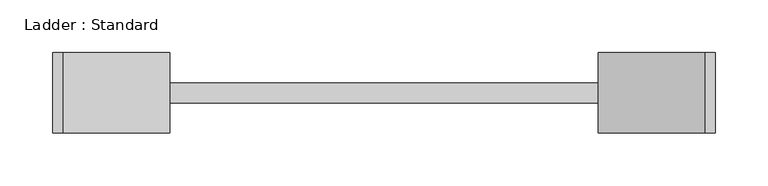
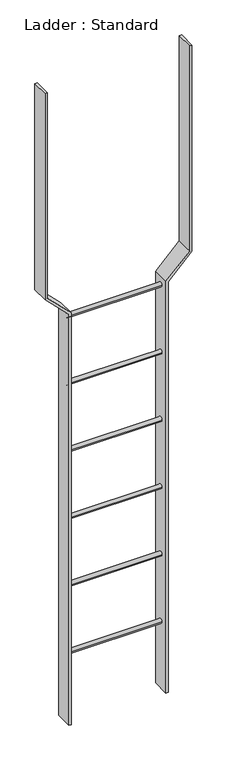
"""IFC4 building model written with IfcOpenShell, lengths in millimetres: proxy geometry, Ladder : Standard."""

from ifc_helpers import new_model, si_unit, point, frame, frame_2d, origin, place, context, project, spatial, polyline, circle_curve, trimmed, segment, composite_curve, outline, extrude, source, transform, mapped, element, save


def ladder_standard_19ab645e(model_context):
    return source(origin(), model_context, "Body", "SweptSolid", [
        extrude(outline(composite_curve([segment(trimmed(circle_curve(frame_2d((102.6687258, -1524.0)), 9.525), [point((93.1437258, -1524.0))], [point((112.1937258, -1524.0))], False, "CARTESIAN"), True, "CONTINUOUS"), segment(trimmed(circle_curve(frame_2d((102.6687258, -1524.0)), 9.525), [point((112.1937258, -1524.0))], [point((93.1437258, -1524.0))], False, "CARTESIAN"), True, "CONTINUOUS")], self_intersect=False)), frame((-203.2, 0.0, 0.0), z_axis=(1.0, 0.0, 0.0), x_axis=(0.0, 1.0, 0.0)), (0.0, 0.0, 1.0), 406.4),
        extrude(outline(composite_curve([segment(trimmed(circle_curve(frame_2d((102.6687258, -1219.2)), 9.525), [point((93.1437258, -1219.2))], [point((112.1937258, -1219.2))], False, "CARTESIAN"), True, "CONTINUOUS"), segment(trimmed(circle_curve(frame_2d((102.6687258, -1219.2)), 9.525), [point((112.1937258, -1219.2))], [point((93.1437258, -1219.2))], False, "CARTESIAN"), True, "CONTINUOUS")], self_intersect=False)), frame((-203.2, 0.0, 0.0), z_axis=(1.0, 0.0, 0.0), x_axis=(0.0, 1.0, 0.0)), (0.0, 0.0, 1.0), 406.4),
        extrude(outline(composite_curve([segment(trimmed(circle_curve(frame_2d((102.6687258, -914.4)), 9.525), [point((93.1437258, -914.4))], [point((112.1937258, -914.4))], False, "CARTESIAN"), True, "CONTINUOUS"), segment(trimmed(circle_curve(frame_2d((102.6687258, -914.4)), 9.525), [point((112.1937258, -914.4))], [point((93.1437258, -914.4))], False, "CARTESIAN"), True, "CONTINUOUS")], self_intersect=False)), frame((-203.2, 0.0, 0.0), z_axis=(1.0, 0.0, 0.0), x_axis=(0.0, 1.0, 0.0)), (0.0, 0.0, 1.0), 406.4),
        extrude(outline(composite_curve([segment(trimmed(circle_curve(frame_2d((102.6687258, -609.6)), 9.525), [point((93.1437258, -609.6))], [point((112.1937258, -609.6))], False, "CARTESIAN"), True, "CONTINUOUS"), segment(trimmed(circle_curve(frame_2d((102.6687258, -609.6)), 9.525), [point((112.1937258, -609.6))], [point((93.1437258, -609.6))], False, "CARTESIAN"), True, "CONTINUOUS")], self_intersect=False)), frame((-203.2, 0.0, 0.0), z_axis=(1.0, 0.0, 0.0), x_axis=(0.0, 1.0, 0.0)), (0.0, 0.0, 1.0), 406.4),
        extrude(outline(composite_curve([segment(trimmed(circle_curve(frame_2d((102.6687258, -304.8)), 9.525), [point((93.1437258, -304.8))], [point((112.1937258, -304.8))], False, "CARTESIAN"), True, "CONTINUOUS"), segment(trimmed(circle_curve(frame_2d((102.6687258, -304.8)), 9.525), [point((112.1937258, -304.8))], [point((93.1437258, -304.8))], False, "CARTESIAN"), True, "CONTINUOUS")], self_intersect=False)), frame((-203.2, 0.0, 0.0), z_axis=(1.0, 0.0, 0.0), x_axis=(0.0, 1.0, 0.0)), (0.0, 0.0, 1.0), 406.4),
        extrude(outline(composite_curve([segment(trimmed(circle_curve(frame_2d((102.6687258, 0.0)), 9.525), [point((93.1437258, 0.0))], [point((112.1937258, 0.0))], False, "CARTESIAN"), True, "CONTINUOUS"), segment(trimmed(circle_curve(frame_2d((102.6687258, 0.0)), 9.525), [point((112.1937258, 0.0))], [point((93.1437258, 0.0))], False, "CARTESIAN"), True, "CONTINUOUS")], self_intersect=False)), frame((-203.2, 0.0, 0.0), z_axis=(1.0, 0.0, 0.0), x_axis=(0.0, 1.0, 0.0)), (0.0, 0.0, 1.0), 406.4),
        extrude(outline(polyline([(1066.8, -314.325), (133.35, -314.325), (31.75, -212.725), (-1828.8, -212.725), (-1828.8, -203.2), (35.6953842, -203.2), (137.2953842, -304.8), (1066.8, -304.8), (1066.8, -314.325)])), frame((0.0, 64.5687258, 0.0), z_axis=(0.0, 1.0, 0.0), x_axis=(0.0, 0.0, 1.0)), (0.0, 0.0, 1.0), 76.2),
        extrude(outline(polyline([(1066.8, 304.8), (137.2953842, 304.8), (35.6953842, 203.2), (-1828.8, 203.2), (-1828.8, 212.725), (31.75, 212.725), (133.35, 314.325), (1066.8, 314.325), (1066.8, 304.8)])), frame((0.0, 64.5687258, 0.0), z_axis=(0.0, 1.0, 0.0), x_axis=(0.0, 0.0, 1.0)), (0.0, 0.0, 1.0), 76.2),
    ])


if __name__ == "__main__":
    model = new_model("IFC4")
    model_context = context("Model", 3, world=origin())
    ifc_project = project(units=[si_unit("LENGTHUNIT", "METRE", prefix="MILLI")], contexts=[model_context])
    site = spatial("IfcSite", under=ifc_project)
    building = spatial("IfcBuilding", under=site)
    placement = place(None, origin())
    ladder_standard_shape = ladder_standard_19ab645e(model_context)
    element("IfcBuildingElementProxy", 1, Name="Ladder : Standard", ObjectType="Ladder : Standard", at=placement, inside=building, context=model_context, shape_type="MappedRepresentation", body=[
        mapped(ladder_standard_shape, transform((0.0, 0.0, 0.0), x_axis=(1.0, 0.0, 0.0), y_axis=(0.0, 1.0, 0.0), z_axis=(0.0, 0.0, 1.0))),
    ])
    save(model, "model.ifc")

# Revit data of these elements
# Type "Ladder : Standard"
#   Rung Radius = 0' - 0 3/8"
#   Rung Length [instance default] = 1' - 4"
#   Side Rail Thickness = 0' - 3"
#   Side Rail Width = 0' - 0 3/8"
#   Half Guardrail Height = 1' - 9"
#   Height [instance default] = 15' - 2 1/2"
#   Guardrail Length = 1' - 8"
#   Guardrail Height = 3' - 6"
#   Distance [instance default] = 0' - 7"
#   Rung Space [instance default] = 1' - 0"
#   Number of Rungs [instance default] = 15
#   Default Elevation = 0
# Element 1 (IfcBuildingElementProxy, "Ladder : Standard")
#   Height = 6' - 0"
#   Distance = 0' - 1.54208"
#   Number of Rungs = 6
